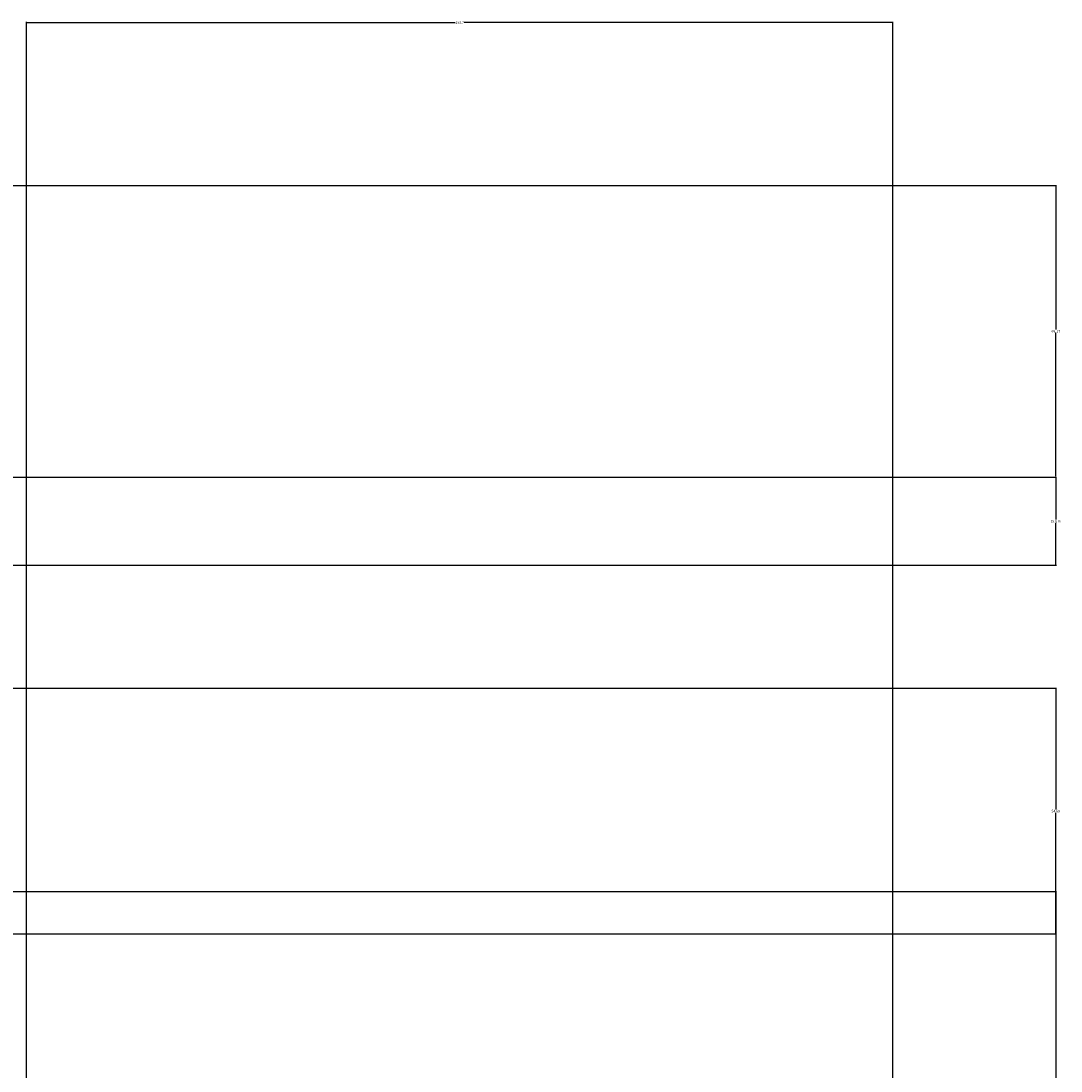
# Model space of a CAD drawing. Units: inches. Extents: x -26 to 776, y -22 to 650.
# Tile 62 of 62: x 544 to 776, y 415 to 650. Entities that reach past the tile are written whole.
import ezdxf

# ---------------------------------------------------------------- set-up
doc = ezdxf.new("R2010")
doc.units = ezdxf.units.IN
doc.header["$MEASUREMENT"] = 0
doc.layers.add('A-ANNO-DIMS', color=2, linetype='Continuous', lineweight=18)
doc.styles.get("Standard").update_dxf_attribs({"font": 'arial.ttf'})
doc.dimstyles.get("Standard").update_dxf_attribs({"dimtxt": 0.5625, "dimasz": 0.18, "dimexe": 0.18, "dimexo": 0.0625, "dimgap": 0.09, "dimtad": 0, "dimtih": 1, "dimtoh": 1, "dimdec": 4, "dimzin": 0, "dimdsep": 46, "dimlunit": 4, "dimtxsty": 'Standard', "dimcen": 0.09, "dimadec": 0, "dimazin": 0, "dimtfac": 1, "dimtdec": 4, "dimtofl": 0, "dimtmove": 0, "dimatfit": 3, "dimfxl": 1, "dimtolj": 1, "dimtzin": 0, "dimarcsym": 0})

# ---------------------------------------------------------------- blocks, each defined once
blk = doc.blocks.new('*D20')
at = {"layer": 'A-ANNO-DIMS', "color": 0, "lineweight": -2, "transparency": 16777216}
for p, q in [((425.81, 455.47), (775.34, 455.47)), ((775.16, 455.29), (775.16, 235.85)), ((775.16, 15.66), (775.16, 235.1)), ((425.81, 15.48), (775.34, 15.48))]:
    blk.add_line(p, q, dxfattribs=at)
at = {"layer": 'A-ANNO-DIMS', "color": 0, "transparency": 16777216}
for points in [[(775.13, 455.29), (775.19, 455.29), (775.16, 455.47)], [(775.13, 15.66), (775.19, 15.66), (775.16, 15.48)]]:
    blk.add_solid(points, dxfattribs=at)
at = {"layer": 'Defpoints', "color": 0, "transparency": 16777216}
for p in [(425.74, 455.47), (775.16, 455.47), (425.74, 15.48)]:
    blk.add_point(p, dxfattribs=at)
at = {"layer": 'A-ANNO-DIMS', "color": 0, "transparency": 16777216, "insert": (775.16, 235.48), "char_height": 0.562, "attachment_point": 5}
blk.add_mtext('\\A1;440', dxfattribs=at)
blk = doc.blocks.new('*D31')
at = {"layer": 'A-ANNO-DIMS', "color": 0, "lineweight": -2, "transparency": 16777216}
for p, q in [((289.3, 500.9), (775.34, 500.9)), ((775.16, 500.72), (775.16, 473.83)), ((775.16, 446.19), (775.16, 473.07)), ((285.08, 446.01), (775.34, 446.01))]:
    blk.add_line(p, q, dxfattribs=at)
at = {"layer": 'A-ANNO-DIMS', "color": 0, "transparency": 16777216}
for points in [[(775.13, 500.72), (775.19, 500.72), (775.16, 500.9)], [(775.13, 446.19), (775.19, 446.19), (775.16, 446.01)]]:
    blk.add_solid(points, dxfattribs=at)
at = {"layer": 'Defpoints', "color": 0, "transparency": 16777216}
for p in [(289.24, 500.9), (775.16, 500.9), (285.02, 446.01)]:
    blk.add_point(p, dxfattribs=at)
at = {"layer": 'A-ANNO-DIMS', "color": 0, "transparency": 16777216, "insert": (775.16, 473.45), "char_height": 0.562, "attachment_point": 5}
blk.add_mtext('\\A1;54.89', dxfattribs=at)
blk = doc.blocks.new('*D32')
at = {"layer": 'A-ANNO-DIMS', "color": 0, "lineweight": -2, "transparency": 16777216}
for p, q in [((357.13, 613.27), (775.34, 613.27)), ((775.16, 613.09), (775.16, 581.06)), ((775.16, 548.28), (775.16, 580.31)), ((357.37, 548.1), (775.34, 548.1))]:
    blk.add_line(p, q, dxfattribs=at)
at = {"layer": 'A-ANNO-DIMS', "color": 0, "transparency": 16777216}
for points in [[(775.13, 613.09), (775.19, 613.09), (775.16, 613.27)], [(775.13, 548.28), (775.19, 548.28), (775.16, 548.1)]]:
    blk.add_solid(points, dxfattribs=at)
at = {"layer": 'Defpoints', "color": 0, "transparency": 16777216}
for p in [(357.07, 613.27), (775.16, 613.27), (357.3, 548.1)]:
    blk.add_point(p, dxfattribs=at)
at = {"layer": 'A-ANNO-DIMS', "color": 0, "transparency": 16777216, "insert": (775.16, 580.69), "char_height": 0.562, "attachment_point": 5}
blk.add_mtext('\\A1;65.17', dxfattribs=at)
blk = doc.blocks.new('*D33')
at = {"layer": 'A-ANNO-DIMS', "color": 0, "lineweight": -2, "transparency": 16777216}
for p, q in [((357.37, 548.1), (775.34, 548.1)), ((775.16, 547.92), (775.16, 538.64)), ((775.16, 528.6), (775.16, 537.88)), ((357.37, 528.42), (775.34, 528.42))]:
    blk.add_line(p, q, dxfattribs=at)
at = {"layer": 'A-ANNO-DIMS', "color": 0, "transparency": 16777216}
for points in [[(775.13, 547.92), (775.19, 547.92), (775.16, 548.1)], [(775.13, 528.6), (775.19, 528.6), (775.16, 528.42)]]:
    blk.add_solid(points, dxfattribs=at)
at = {"layer": 'Defpoints', "color": 0, "transparency": 16777216}
for p in [(357.3, 548.1), (775.16, 548.1), (357.3, 528.42)]:
    blk.add_point(p, dxfattribs=at)
at = {"layer": 'A-ANNO-DIMS', "color": 0, "transparency": 16777216, "insert": (775.16, 538.26), "char_height": 0.562, "attachment_point": 5}
blk.add_mtext('\\A1;19.676', dxfattribs=at)
blk = doc.blocks.new('*D48')
at = {"layer": 'A-ANNO-DIMS', "color": 0, "lineweight": -2, "transparency": 16777216}
for p, q in [((545.03, 67.41), (545.03, 649.86)), ((545.21, 649.68), (640.88, 649.68)), ((738.57, 649.68), (642.9, 649.68)), ((738.75, 50.91), (738.75, 649.86))]:
    blk.add_line(p, q, dxfattribs=at)
at = {"layer": 'A-ANNO-DIMS', "color": 0, "transparency": 16777216}
for points in [[(545.21, 649.71), (545.21, 649.65), (545.03, 649.68)], [(738.57, 649.71), (738.57, 649.65), (738.75, 649.68)]]:
    blk.add_solid(points, dxfattribs=at)
at = {"layer": 'Defpoints', "color": 0, "transparency": 16777216}
for p in [(738.75, 649.68), (545.03, 67.35), (738.75, 50.85)]:
    blk.add_point(p, dxfattribs=at)
at = {"layer": 'A-ANNO-DIMS', "color": 0, "transparency": 16777216, "insert": (641.89, 649.68), "char_height": 0.562, "attachment_point": 5}
blk.add_mtext('\\A1;193.7', dxfattribs=at)

msp = doc.modelspace()

# ---------------------------------------------------------------- dimensions: what is measured, and where the dimension line sits
at = {"layer": 'A-ANNO-DIMS'}
dim = msp.add_linear_dim(base=(738.7503, 649.6763), p1=(545.0331, 67.3523), p2=(738.7503, 50.8482), dimstyle='Standard', override={"dimdec": 1, "dimlfac": 1, "dimrnd": 0, "dimzin": 0, "dimdsep": 46, "dimlunit": 2}, dxfattribs=at)
dim.commit()
dim.dimension.update_dxf_attribs({"geometry": '*D48', "text_midpoint": (641.8917, 649.6763)})
for base, p1, p2, override, picture, middle in [((775.1553, 613.2713), (357.3034, 548.0996), (357.0669, 613.2713), {"dimdec": 2, "dimlfac": 1, "dimrnd": 0, "dimzin": 0, "dimdsep": 46, "dimlunit": 2}, '*D32', (775.1553, 580.6855)), ((775.1553, 548.0996), (357.3034, 528.4233), (357.3034, 548.0996), {"dimdec": 3, "dimlfac": 1, "dimrnd": 0, "dimzin": 0, "dimdsep": 46, "dimlunit": 2}, '*D33', (775.1553, 538.2614)), ((775.1553, 500.896), (285.0179, 446.0063), (289.2424, 500.896), {"dimdec": 2, "dimlfac": 1, "dimrnd": 0, "dimzin": 0, "dimdsep": 46, "dimlunit": 2}, '*D31', (775.1553, 473.4511)), ((775.1553, 455.4717), (425.7434, 15.4824), (425.7434, 455.4717), {"dimdec": 0, "dimlfac": 1, "dimrnd": 0, "dimzin": 0, "dimdsep": 46, "dimlunit": 2}, '*D20', (775.1553, 235.477))]:
    dim = msp.add_linear_dim(base=base, p1=p1, p2=p2, angle=90, dimstyle='Standard', override=override, dxfattribs=at)
    dim.commit()
    dim.dimension.update_dxf_attribs({"geometry": picture, "text_midpoint": middle})

doc.saveas('drawing.dxf')
